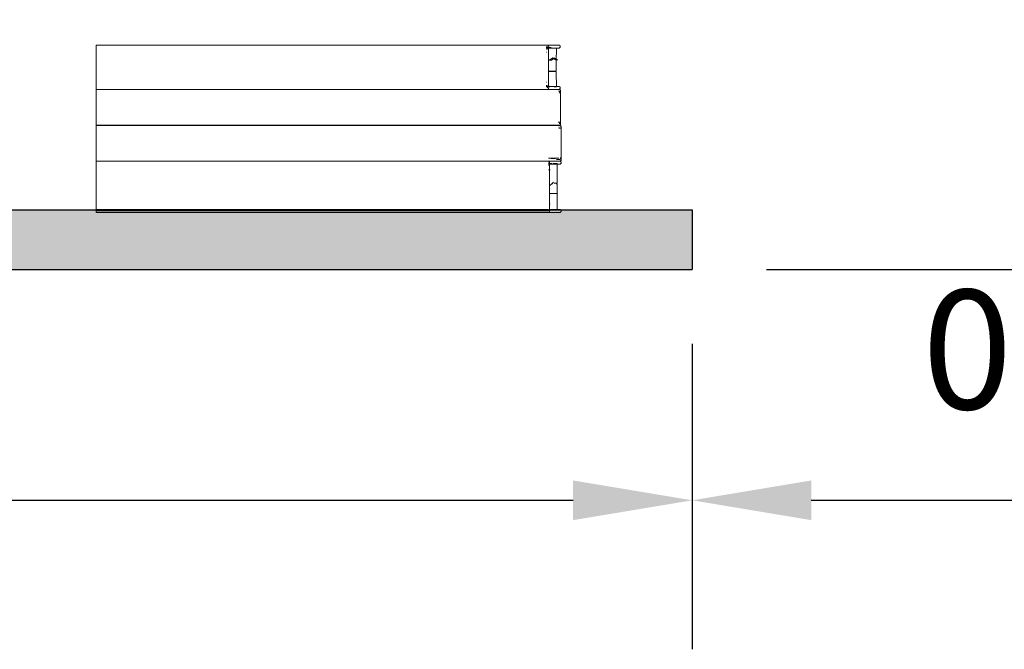
# Model space of a CAD drawing. Units: millimetres. Extents: x 7894 to 8038, y 6851 to 6951.
# Tile 25 of 49: x 7958.696 to 7966.961, y 6903.287 to 6908.569. Entities that reach past the tile are written whole.
import ezdxf

# ---------------------------------------------------------------- set-up
doc = ezdxf.new("R2010")
doc.units = ezdxf.units.MM
for name, color, linetype, lineweight in [('A-ANNO-DIMS', 2, 'Continuous', 18), ('A-FURN-BOOK', 8, 'Continuous', 13), ('A-FURN-SHLF', 7, 'Continuous', 30)]:
    doc.layers.add(name, color=color, linetype=linetype, lineweight=lineweight)
doc.layers.add('A-FURN-PATT', color=32, linetype='Continuous', lineweight=9, true_color=0xcd6928)
doc.styles.get("Standard").update_dxf_attribs({"font": 'arial.ttf'})
doc.dimstyles.new('ISO-25', dxfattribs={"dimtxt": 1, "dimasz": 1, "dimexe": 1.25, "dimexo": 0.625, "dimtad": 1, "dimdec": 0, "dimlunit": 4, "dimtxsty": 'Standard', "dimcen": 2.5, "dimclrt": 1, "dimadec": 0, "dimazin": 0, "dimtfac": 1, "dimtdec": 0, "dimtmove": 0, "dimatfit": 3, "dimfxl": 1, "dimarcsym": 0})

# ---------------------------------------------------------------- blocks, each defined once
blk = doc.blocks.new('*D23')
at = {"layer": 'A-ANNO-DIMS', "color": 0, "lineweight": -2, "transparency": 16777216}
for p, q in [((7940.0888, 6907.098), (7940.0888, 6947.7928)), ((7971.9356, 6928.989), (7971.9356, 6947.7928)), ((7941.0888, 6946.5428), (7970.9356, 6946.5428))]:
    blk.add_line(p, q, dxfattribs=at)
at = {"layer": 'A-ANNO-DIMS', "color": 0, "transparency": 16777216}
for points in [[(7941.0888, 6946.7095), (7941.0888, 6946.3762), (7940.0888, 6946.5428)], [(7970.9356, 6946.7095), (7970.9356, 6946.3762), (7971.9356, 6946.5428)]]:
    blk.add_solid(points, dxfattribs=at)
at = {"layer": 'Defpoints', "color": 0, "transparency": 16777216}
for p in [(7971.9356, 6946.5428), (7971.9356, 6928.364), (7940.0888, 6906.473)]:
    blk.add_point(p, dxfattribs=at)
at = {"layer": 'A-ANNO-DIMS', "color": 1, "transparency": 16777216, "insert": (7956.0122, 6947.6784), "char_height": 1, "attachment_point": 5}
blk.add_mtext('2\'-8"', dxfattribs=at)
blk = doc.blocks.new('*D25')
at = {"layer": 'A-ANNO-DIMS', "color": 0, "lineweight": -2, "transparency": 16777216}
for p, q in [((7940.0888, 6905.848), (7940.0888, 6903.2865)), ((7964.3408, 6905.8484), (7964.3408, 6903.2865)), ((7941.0888, 6904.5365), (7963.3408, 6904.5365))]:
    blk.add_line(p, q, dxfattribs=at)
at = {"layer": 'A-ANNO-DIMS', "color": 0, "transparency": 16777216}
for points in [[(7941.0888, 6904.7032), (7941.0888, 6904.3699), (7940.0888, 6904.5365)], [(7963.3408, 6904.7032), (7963.3408, 6904.3699), (7964.3408, 6904.5365)]]:
    blk.add_solid(points, dxfattribs=at)
at = {"layer": 'Defpoints', "color": 0, "transparency": 16777216}
for p in [(7940.0888, 6906.473), (7964.3408, 6906.4734), (7964.3408, 6904.5365)]:
    blk.add_point(p, dxfattribs=at)
at = {"layer": 'A-ANNO-DIMS', "color": 1, "transparency": 16777216, "insert": (7952.2148, 6905.6786), "char_height": 1, "attachment_point": 5}
blk.add_mtext('2\'-0 1/2"', dxfattribs=at)
blk = doc.blocks.new('*D26')
at = {"layer": 'A-ANNO-DIMS', "color": 0, "lineweight": -2, "transparency": 16777216}
for p, q in [((7950.9654, 6918.7198), (7975.2272, 6918.7198)), ((7973.9772, 6917.7198), (7973.9772, 6907.4734)), ((7964.9658, 6906.4734), (7975.2272, 6906.4734))]:
    blk.add_line(p, q, dxfattribs=at)
at = {"layer": 'A-ANNO-DIMS', "color": 0, "transparency": 16777216}
for points in [[(7973.8105, 6917.7198), (7974.1439, 6917.7198), (7973.9772, 6918.7198)], [(7973.8105, 6907.4734), (7974.1439, 6907.4734), (7973.9772, 6906.4734)]]:
    blk.add_solid(points, dxfattribs=at)
at = {"layer": 'Defpoints', "color": 0, "transparency": 16777216}
for p in [(7950.3404, 6918.7198), (7964.3408, 6906.4734), (7973.9772, 6906.4734)]:
    blk.add_point(p, dxfattribs=at)
at = {"layer": 'A-ANNO-DIMS', "color": 1, "transparency": 16777216, "insert": (7972.8416, 6912.5966), "char_height": 1, "attachment_point": 5, "rotation": 90}
blk.add_mtext('1\'-0"', dxfattribs=at)
blk = doc.blocks.new('*D34')
at = {"layer": 'A-ANNO-DIMS', "color": 0, "lineweight": -2, "transparency": 16777216}
for p, q in [((7971.2171, 6922.0033), (7971.2171, 6903.2865)), ((7964.3408, 6905.8484), (7964.3408, 6903.2865)), ((7965.3408, 6904.5365), (7970.2171, 6904.5365))]:
    blk.add_line(p, q, dxfattribs=at)
at = {"layer": 'A-ANNO-DIMS', "color": 0, "transparency": 16777216}
for points in [[(7965.3408, 6904.7032), (7965.3408, 6904.3699), (7964.3408, 6904.5365)], [(7970.2171, 6904.7032), (7970.2171, 6904.3699), (7971.2171, 6904.5365)]]:
    blk.add_solid(points, dxfattribs=at)
at = {"layer": 'Defpoints', "color": 0, "transparency": 16777216}
for p in [(7971.2171, 6922.6283), (7964.3408, 6906.4734), (7971.2171, 6904.5365)]:
    blk.add_point(p, dxfattribs=at)
at = {"layer": 'A-ANNO-DIMS', "color": 1, "transparency": 16777216, "insert": (7967.779, 6905.6721), "char_height": 1, "attachment_point": 5}
blk.add_mtext('0\'-7"', dxfattribs=at)

msp = doc.modelspace()

# ---------------------------------------------------------------- hatches: boundary and pattern name
at = {"layer": 'A-FURN-PATT'}
h = msp.add_hatch(color=256, dxfattribs=at)
h.dxf.hatch_style = 1
h.paths.add_polyline_path([(7942.8406, 6913.3629), (7942.8593, 6913.356), (7942.8677, 6913.356), (7942.8677, 6914.2132), (7942.876, 6914.2376), (7942.8813, 6914.2376), (7942.9022, 6914.2457), (7943.3657, 6914.2457), (7943.3844, 6914.2376), (7943.3861, 6914.2376), (7943.3858, 6914.2132), (7943.3852, 6913.2312), (7943.3944, 6906.9948), (7943.387, 6906.9732), (7943.4027, 6906.9732), (7943.403, 6906.9948), (7943.4029, 6908.4372), (7943.3944, 6914.2132), (7943.4169, 6914.2376), (7943.4198, 6914.2457), (7943.4555, 6914.2457), (7943.4603, 6914.238), (7943.8607, 6914.2452), (7943.8615, 6914.2457), (7943.8623, 6914.2452), (7943.8866, 6914.2457), (7943.8944, 6914.2402), (7943.9104, 6914.2376), (7943.9211, 6914.2132), (7943.9294, 6914.2376), (7943.9318, 6914.2376), (7943.9453, 6914.2398), (7943.9488, 6914.2457), (7943.9797, 6914.2452), (7943.9807, 6914.2457), (7943.9815, 6914.2451), (7944.3738, 6914.2376), (7944.3882, 6914.2457), (7944.4201, 6914.2457), (7944.4341, 6914.2376), (7944.4395, 6914.2376), (7944.4478, 6914.2132), (7944.4478, 6914.1031), (7944.4622, 6914.099), (7944.7359, 6914.1607), (7944.8923, 6914.2014), (7944.9541, 6914.2098), (7944.955, 6914.21), (7946.556, 6907.1325), (7946.5534, 6907.1122), (7946.5529, 6907.1152), (7946.499, 6907.103), (7946.3343, 6907.0604), (7946.0282, 6906.9914), (7945.6731, 6908.5712), (7944.4484, 6914.0015), (7944.4478, 6906.9948), (7944.4404, 6906.9732), (7947.0373, 6906.9734), (7964.3408, 6906.9734), (7964.3408, 6906.4734), (7947.0373, 6906.4734), (7940.0888, 6906.473), (7940.0888, 6906.973), (7941.9951, 6906.9731), (7941.9899, 6906.9898), (7941.9899, 6913.3353), (7941.9968, 6913.3574), (7942.003, 6913.3571), (7942.0169, 6913.3629), (7942.0366, 6913.3629), (7942.0378, 6913.3629), (7942.0479, 6913.356), (7942.8142, 6913.356), (7942.8157, 6913.356), (7942.8346, 6913.356)])
h.paths.add_polyline_path([(7942.8598, 6913.0201), (7942.861, 6913.3353), (7942.8677, 6906.9948), (7942.876, 6906.9759), (7942.876, 6906.9903), (7942.8813, 6914.2376), (7942.876, 6914.2321), (7942.876, 6914.2177), (7942.8809, 6906.9647), (7942.8784, 6906.9704), (7942.876, 6906.9704), (7942.8574, 6906.9704), (7942.8613, 6911.8549)], flags=16)
h.paths.add_polyline_path([(7942.8613, 6911.8549), (7942.8677, 6906.9948), (7942.8686, 6906.9921), (7942.8677, 6906.9898), (7942.8616, 6906.9704), (7942.8598, 6906.9704), (7942.8574, 6906.9704), (7942.0002, 6906.9704), (7941.9978, 6906.9704), (7941.996, 6906.9704), (7941.9899, 6906.9898), (7941.9978, 6906.9704), (7942.0002, 6906.9704), (7942.8598, 6906.9704), (7942.8616, 6906.9748)], flags=16)
h.paths.add_polyline_path([(7942.023, 6913.356), (7942.0169, 6913.3629), (7942.0366, 6913.3629), (7942.0378, 6913.3629), (7942.0367, 6913.3614), (7942.0369, 6913.356)], flags=16)
h.paths.add_polyline_path([(7942.0366, 6913.3629), (7942.0169, 6913.3629), (7942.0196, 6913.3598)], flags=0)
h.paths.add_polyline_path([(7942.0353, 6913.356), (7942.0369, 6913.356), (7942.0367, 6913.3614)], flags=0)
h.paths.add_polyline_path([(7943.9293, 6906.9759), (7943.9211, 6906.9948), (7943.9294, 6906.9704)], flags=0)
h.paths.add_polyline_path([(7943.9125, 6914.2132), (7943.8982, 6914.2376), (7943.8944, 6914.2402), (7943.8832, 6914.2421), (7943.8781, 6914.2367), (7943.8765, 6914.2376), (7943.8789, 6914.2376), (7943.8866, 6914.2457), (7943.8623, 6914.2452), (7943.8607, 6914.2452), (7943.8615, 6914.2457), (7943.8623, 6914.2452), (7943.8866, 6914.2457), (7943.8944, 6914.2402), (7943.8982, 6914.2376), (7943.9097, 6914.218), (7943.9125, 6914.2168), (7943.9079, 6906.9704), (7943.9104, 6906.9704), (7943.9211, 6914.2132), (7943.9294, 6914.2376), (7943.9318, 6914.2376), (7943.9453, 6914.2398), (7943.9488, 6914.2457), (7943.9797, 6914.2452), (7943.9807, 6914.2457), (7943.9815, 6914.2451), (7944.3738, 6914.2376), (7944.3882, 6914.2457), (7944.4201, 6914.2457), (7944.4341, 6914.2376), (7944.4395, 6914.2376), (7944.4395, 6914.2177), (7944.4341, 6914.0941), (7944.4478, 6914.1004), (7944.4513, 6914.1021), (7944.4622, 6914.099), (7944.4343, 6914.0927), (7944.429, 6914.0915), (7944.4341, 6914.069), (7944.4484, 6914.0015), (7944.4341, 6914.0649), (7944.4346, 6906.9704), (7944.4371, 6906.9704), (7944.4395, 6906.9759), (7944.4395, 6906.9704), (7943.931, 6906.9704), (7943.9128, 6906.9704), (7943.9079, 6906.9704)], flags=16)
h.paths.add_polyline_path([(7943.9211, 6914.2132), (7943.9294, 6914.2376), (7943.9318, 6914.2376), (7943.9453, 6914.2398), (7943.9488, 6914.2457), (7943.9797, 6914.2452), (7943.9807, 6914.2457), (7943.9815, 6914.2451), (7944.3738, 6914.2376), (7944.3882, 6914.2457), (7944.4201, 6914.2457), (7944.4321, 6914.2387), (7944.4249, 6914.2376), (7944.4041, 6914.2376), (7944.4032, 6914.2136), (7944.4032, 6914.2376), (7944.4025, 6914.2379), (7944.3897, 6914.2382), (7944.3753, 6914.2384), (7944.3738, 6914.2376), (7943.9815, 6914.2451), (7943.9488, 6914.2457), (7943.9453, 6914.2398), (7943.9294, 6914.2132), (7943.931, 6906.9721), (7943.931, 6906.9704), (7943.9294, 6906.9704), (7943.9293, 6906.9759), (7943.9294, 6914.2132), (7943.9439, 6914.2376), (7943.9318, 6914.2376)], flags=0)
h.paths.add_polyline_path([(7942.8813, 6914.2376), (7942.8778, 6914.2362), (7942.8796, 6914.2404), (7942.885, 6914.239)], flags=17)
h.paths.add_polyline_path([(7944.4116, 6914.242), (7944.4104, 6914.2408), (7944.4125, 6914.2418)], flags=0)
h.paths.add_polyline_path([(7944.3879, 6914.2382), (7944.3882, 6914.2457), (7944.4094, 6914.241), (7944.4103, 6914.2408), (7944.4036, 6914.2373), (7944.39, 6914.2447), (7944.3897, 6914.2382)], flags=0)
h.paths.add_polyline_path([(7963.1359, 6906.9526), (7963.1396, 6906.9526), (7963.1431, 6906.9582)], flags=16)
h.paths.add_polyline_path([(7954.3975, 6907.3902), (7954.397, 6907.3948), (7954.3984, 6907.4007), (7954.3975, 6907.567), (7954.3984, 6907.5978), (7954.3986, 6907.7694), (7954.3978, 6907.7989), (7954.399, 6907.8759), (7954.3992, 6907.9037), (7954.3944, 6907.9081), (7954.4019, 6907.9055), (7954.3996, 6907.93), (7954.3988, 6907.9307), (7954.3841, 6907.9429), (7946.6754, 6907.9429), (7946.6535, 6907.9232), (7946.6531, 6907.9127), (7946.6527, 6907.7694), (7946.6525, 6907.4007), (7946.653, 6907.1185), (7946.6574, 6907.1224), (7946.656, 6907.1145), (7946.6571, 6907.1135), (7946.6675, 6907.1209), (7946.7515, 6907.1209), (7946.9105, 6907.1209), (7954.3003, 6907.1209), (7954.3895, 6907.1209), (7954.3915, 6907.1191), (7954.3991, 6907.1209), (7954.399, 6907.1383), (7954.3978, 6907.2163), (7954.3986, 6907.2413)], flags=17)
h.paths.add_polyline_path([(7954.3003, 6907.1209), (7954.3003, 6907.1136), (7946.9105, 6907.1129), (7946.7516, 6907.1136), (7946.7515, 6907.1209), (7946.6675, 6907.1209), (7946.6531, 6907.1106), (7946.653, 6907.1185), (7946.6574, 6907.1224), (7946.656, 6907.1145), (7946.6571, 6907.1135), (7946.6675, 6907.1209), (7946.7515, 6907.1209), (7946.9105, 6907.1209)], flags=17)
h.paths.add_polyline_path([(7954.3981, 6907.9048), (7954.3944, 6907.9081), (7954.3997, 6907.9062), (7954.4007, 6907.9186), (7954.4019, 6907.9055), (7954.405, 6907.9072), (7954.4044, 6907.9046), (7954.4027, 6907.8974), (7954.4024, 6907.9009), (7954.3996, 6907.9034), (7954.3996, 6907.9025), (7954.3994, 6907.9023), (7954.3995, 6907.9035)], flags=17)

# ---------------------------------------------------------------- linework, layer by layer
at = {"layer": 'A-FURN-BOOK'}
for p, q in [((7963.1286, 6908.3556), (7959.3384, 6908.3556)), ((7959.3384, 6906.9526), (7959.3384, 6908.3556)), ((7963.1316, 6908.353), (7963.1286, 6908.3556)), ((7963.2254, 6908.3556), (7963.1286, 6908.3556)), ((7963.1316, 6908.353), (7963.1358, 6908.35)), ((7963.1358, 6908.3494), (7963.1358, 6908.35)), ((7963.1363, 6908.349), (7963.1358, 6908.3494)), ((7963.1367, 6908.3434), (7963.1363, 6908.349)), ((7963.2254, 6908.3556), (7963.233, 6908.3486)), ((7963.233, 6908.3486), (7963.233, 6908.3376)), ((7963.1299, 6908.3414), (7963.1163, 6908.3414)), ((7963.1172, 6908.3363), (7963.1163, 6908.3366)), ((7963.1163, 6908.3305), (7963.1276, 6908.3305)), ((7963.1183, 6908.3228), (7963.1163, 6908.3228)), ((7963.1169, 6908.2977), (7963.1163, 6908.2977)), ((7963.1324, 6908.3366), (7963.1172, 6908.3363)), ((7963.1287, 6908.3295), (7963.1276, 6908.3295)), ((7963.1299, 6908.3228), (7963.1276, 6908.3228)), ((7963.1293, 6908.3299), (7963.1287, 6908.3295)), ((7963.1336, 6908.338), (7963.1299, 6908.3414)), ((7963.1359, 6908.3283), (7963.1299, 6908.3228)), ((7963.1354, 6908.3363), (7963.1362, 6908.3364)), ((7963.1362, 6908.3356), (7963.1354, 6908.3363)), ((7963.1362, 6908.3352), (7963.1354, 6908.3346)), ((7963.1354, 6908.3305), (7963.1362, 6908.3352)), ((7963.1359, 6908.3298), (7963.1354, 6908.3305)), ((7963.136, 6908.3305), (7963.1354, 6908.3305)), ((7963.1354, 6908.2332), (7963.1358, 6908.2861)), ((7963.1358, 6908.2861), (7963.1359, 6908.3217)), ((7963.1359, 6908.3283), (7963.1359, 6908.3298)), ((7963.1375, 6908.3298), (7963.1359, 6908.3283)), ((7963.1359, 6908.3217), (7963.1359, 6908.3283)), ((7963.1378, 6908.3301), (7963.136, 6908.3305)), ((7963.1362, 6908.3364), (7963.1367, 6908.3434)), ((7963.1362, 6908.3364), (7963.1373, 6908.3367)), ((7963.1362, 6908.3356), (7963.1362, 6908.3364)), ((7963.1375, 6908.3344), (7963.1362, 6908.3356)), ((7963.1362, 6908.3352), (7963.1362, 6908.3356)), ((7963.1373, 6908.3367), (7963.1367, 6908.3434)), ((7963.1388, 6908.3376), (7963.1373, 6908.3367)), ((7963.1373, 6908.3367), (7963.1386, 6908.3365)), ((7963.1375, 6908.3344), (7963.1373, 6908.3367)), ((7963.1375, 6908.3298), (7963.1378, 6908.3301)), ((7963.1378, 6908.3301), (7963.138, 6908.3319)), ((7963.1378, 6908.3301), (7963.1405, 6908.3305)), ((7963.138, 6908.3319), (7963.1384, 6908.3357)), ((7963.1384, 6908.3357), (7963.1386, 6908.3365)), ((7963.1386, 6908.3365), (7963.1388, 6908.3376)), ((7963.1386, 6908.3365), (7963.1402, 6908.3366)), ((7963.1405, 6908.3305), (7963.2012, 6908.3305)), ((7963.1443, 6908.3364), (7963.1427, 6908.3366)), ((7963.1583, 6908.3366), (7963.1443, 6908.3364)), ((7963.2009, 6908.2977), (7963.2006, 6908.2549)), ((7963.2012, 6908.3305), (7963.2009, 6908.2977)), ((7963.2012, 6908.3305), (7963.2254, 6908.3305)), ((7963.233, 6908.3376), (7963.2254, 6908.3305)), ((7963.1358, 6908.2327), (7963.1354, 6908.2332)), ((7963.1354, 6908.2327), (7963.1354, 6908.2332)), ((7963.1354, 6908.2327), (7963.1358, 6908.2327)), ((7963.1354, 6908.2314), (7963.1354, 6908.2327)), ((7963.1354, 6908.2314), (7963.1358, 6908.2314)), ((7963.1354, 6908.2307), (7963.1354, 6908.2314)), ((7963.1354, 6908.2307), (7963.1467, 6908.2308)), ((7963.1354, 6908.2295), (7963.1354, 6908.2307)), ((7963.1354, 6908.2295), (7963.1358, 6908.229)), ((7963.1354, 6908.229), (7963.1354, 6908.2295)), ((7963.1358, 6908.229), (7963.1354, 6908.229)), ((7963.1358, 6908.2103), (7963.1354, 6908.229)), ((7963.1354, 6908.1368), (7963.1358, 6908.2103)), ((7963.1431, 6908.2332), (7963.1358, 6908.2327)), ((7963.1358, 6908.2314), (7963.1467, 6908.2308)), ((7963.1436, 6908.2291), (7963.1358, 6908.229)), ((7963.1431, 6908.2332), (7963.1436, 6908.2328)), ((7963.1436, 6908.2328), (7963.1444, 6908.2332)), ((7963.1444, 6908.2295), (7963.1436, 6908.2291)), ((7963.145, 6908.2332), (7963.1444, 6908.2332)), ((7963.1588, 6908.2309), (7963.1444, 6908.2295)), ((7963.1467, 6908.2308), (7963.1444, 6908.2295)), ((7963.145, 6908.2332), (7963.1707, 6908.2484)), ((7963.1467, 6908.2308), (7963.1472, 6908.2314)), ((7963.1588, 6908.2309), (7963.1472, 6908.2314)), ((7963.1707, 6908.2446), (7963.1585, 6908.2376)), ((7963.1588, 6908.2309), (7963.177, 6908.2414)), ((7963.1859, 6908.2465), (7963.1707, 6908.2484)), ((7963.1707, 6908.2484), (7963.1766, 6908.2453)), ((7963.1766, 6908.2453), (7963.1707, 6908.2446)), ((7963.1743, 6908.2427), (7963.1707, 6908.2446)), ((7963.1859, 6908.2465), (7963.1766, 6908.2453)), ((7963.1766, 6908.2453), (7963.1789, 6908.2442)), ((7963.177, 6908.2414), (7963.1805, 6908.2434)), ((7963.1931, 6908.2332), (7963.177, 6908.2414)), ((7963.1805, 6908.2434), (7963.1859, 6908.2465)), ((7963.1805, 6908.2434), (7963.1948, 6908.2362)), ((7963.2006, 6908.2382), (7963.1859, 6908.2465)), ((7963.1973, 6908.2332), (7963.1931, 6908.2332)), ((7963.1968, 6908.2314), (7963.1931, 6908.2332)), ((7963.1968, 6908.2314), (7963.1989, 6908.2314)), ((7963.2005, 6908.2295), (7963.1968, 6908.2314)), ((7963.2126, 6908.2314), (7963.2005, 6908.2295)), ((7963.2005, 6908.2295), (7963.2005, 6908.2078)), ((7963.2005, 6908.1368), (7963.2005, 6908.2078)), ((7963.2006, 6908.2549), (7963.2006, 6908.2382)), ((7963.2126, 6908.2314), (7963.2006, 6908.2382)), ((7963.1354, 6908.133), (7963.1354, 6908.1368)), ((7963.1354, 6908.1368), (7963.1436, 6908.1368)), ((7963.1358, 6908.1255), (7963.1354, 6908.133)), ((7963.1358, 6908.133), (7963.1354, 6908.133)), ((7963.1358, 6908.133), (7963.1436, 6908.1331)), ((7963.1358, 6908.1255), (7963.1359, 6908.0187)), ((7963.1436, 6908.1368), (7963.2005, 6908.1368)), ((7963.1436, 6908.1331), (7963.2005, 6908.133)), ((7963.2005, 6908.1368), (7963.1763, 6908.1349)), ((7963.1763, 6908.1349), (7963.2005, 6908.133)), ((7963.2006, 6908.0878), (7963.2005, 6908.133)), ((7963.1163, 6908.0451), (7963.1169, 6908.0451)), ((7963.1256, 6908.0177), (7963.1163, 6908.0177)), ((7963.1359, 6908.0121), (7963.1359, 6908.0187)), ((7963.2006, 6908.0878), (7963.2009, 6908.0451)), ((7963.2009, 6908.0451), (7963.2018, 6908.0099)), ((7963.1286, 6907.9848), (7959.3384, 6907.9848)), ((7963.2269, 6907.9836), (7959.4277, 6907.9836)), ((7963.1278, 6908.0109), (7963.1163, 6908.0109)), ((7963.1163, 6908.0099), (7963.1301, 6908.0099)), ((7963.1191, 6908.0064), (7963.1323, 6908.0061)), ((7963.1323, 6908.0061), (7963.1193, 6908.0061)), ((7963.1291, 6907.999), (7963.1251, 6907.999)), ((7963.1286, 6907.9848), (7963.1358, 6907.9905)), ((7963.1286, 6907.9848), (7963.2254, 6907.9848)), ((7963.1301, 6908.0099), (7963.1293, 6908.0105)), ((7963.1312, 6908.0099), (7963.1301, 6908.0099)), ((7963.1312, 6908.0099), (7963.1332, 6908.008)), ((7963.133, 6908.0076), (7963.1312, 6908.0099)), ((7963.1341, 6908.0099), (7963.1312, 6908.0099)), ((7963.1359, 6908.0121), (7963.1352, 6908.0128)), ((7963.1354, 6908.0099), (7963.1359, 6908.0106)), ((7963.136, 6908.0099), (7963.1354, 6908.0099)), ((7963.1354, 6908.0063), (7963.1354, 6908.0099)), ((7963.1354, 6908.0063), (7963.1362, 6908.006)), ((7963.1362, 6908.006), (7963.1354, 6908.006)), ((7963.1362, 6908.0048), (7963.1354, 6908.0041)), ((7963.1358, 6907.9905), (7963.1363, 6907.9913)), ((7963.1359, 6908.0106), (7963.1359, 6908.0121)), ((7963.1375, 6908.0106), (7963.1359, 6908.0121)), ((7963.1378, 6908.0103), (7963.136, 6908.0099)), ((7963.1362, 6908.0052), (7963.1362, 6908.006)), ((7963.1375, 6908.006), (7963.1362, 6908.0052)), ((7963.1375, 6908.006), (7963.1362, 6908.006)), ((7963.1362, 6908.0052), (7963.1362, 6908.0048)), ((7963.1362, 6908.0048), (7963.1367, 6907.9965)), ((7963.1362, 6908.0048), (7963.1373, 6908.0039)), ((7963.1363, 6907.9913), (7963.1367, 6907.9965)), ((7963.1367, 6907.9965), (7963.1373, 6908.0039)), ((7963.1373, 6908.0039), (7963.1375, 6908.006)), ((7963.1373, 6908.0039), (7963.1388, 6908.0028)), ((7963.1378, 6908.0103), (7963.1375, 6908.0106)), ((7963.1405, 6908.0099), (7963.1378, 6908.0103)), ((7963.138, 6908.0084), (7963.1378, 6908.0103)), ((7963.1384, 6908.0048), (7963.138, 6908.0084)), ((7963.1388, 6908.0028), (7963.1384, 6908.0048)), ((7963.2018, 6908.0099), (7963.1405, 6908.0099)), ((7963.182, 6908.0062), (7963.1825, 6908.0061)), ((7963.2013, 6908.0061), (7963.1825, 6908.0061)), ((7963.2018, 6908.0099), (7963.2013, 6908.0061)), ((7963.2018, 6908.0099), (7963.2254, 6908.0099)), ((7963.2269, 6907.9698), (7963.2182, 6907.9698)), ((7963.2254, 6908.0099), (7963.233, 6908.0028)), ((7963.233, 6907.9918), (7963.2254, 6907.9848)), ((7963.2269, 6907.9836), (7963.2345, 6907.9768)), ((7963.2345, 6907.9772), (7963.2269, 6907.9836)), ((7963.2269, 6907.9836), (7963.2345, 6907.9781)), ((7963.2326, 6907.9646), (7963.2269, 6907.9698)), ((7963.2326, 6907.9646), (7963.2269, 6907.9592)), ((7963.2341, 6907.9633), (7963.2269, 6907.9582)), ((7963.2345, 6907.9584), (7963.2269, 6907.9516)), ((7963.2345, 6907.9663), (7963.2326, 6907.9646)), ((7963.2341, 6907.9633), (7963.2326, 6907.9646)), ((7963.233, 6908.0028), (7963.233, 6907.9918)), ((7963.2341, 6907.9633), (7963.2345, 6907.9642)), ((7963.2345, 6907.9636), (7963.2341, 6907.9633)), ((7963.2345, 6907.9629), (7963.2341, 6907.9633)), ((7963.2345, 6907.9772), (7963.2345, 6907.9781)), ((7963.2345, 6907.9768), (7963.2345, 6907.9772)), ((7963.2345, 6907.9663), (7963.2345, 6907.9768)), ((7963.2345, 6907.9642), (7963.2345, 6907.9663)), ((7963.2345, 6907.9642), (7963.2345, 6907.9636)), ((7963.2345, 6907.9636), (7963.2345, 6907.9629)), ((7963.2345, 6907.9632), (7963.2345, 6907.9636)), ((7963.2345, 6907.9629), (7963.2345, 6907.9632)), ((7963.2345, 6907.9584), (7963.2345, 6907.9629)), ((7963.2345, 6907.9584), (7963.2345, 6907.6896)), ((7963.2156, 6907.7085), (7963.2269, 6907.7085)), ((7963.2269, 6907.6979), (7963.2243, 6907.6979)), ((7963.2282, 6907.7149), (7963.2269, 6907.716)), ((7963.2269, 6907.7085), (7963.2313, 6907.7045)), ((7963.2293, 6907.7001), (7963.2269, 6907.6979)), ((7963.2345, 6907.6896), (7963.2269, 6907.684)), ((7963.232, 6907.7058), (7963.2278, 6907.7088)), ((7963.2338, 6907.7098), (7963.2328, 6907.7107)), ((7963.2269, 6907.684), (7959.3384, 6907.684)), ((7959.3384, 6907.6826), (7963.2304, 6907.6826)), ((7963.2253, 6907.6687), (7963.2228, 6907.6687)), ((7963.2304, 6907.6582), (7963.2229, 6907.6582)), ((7963.2304, 6907.6826), (7963.2337, 6907.6796)), ((7963.2336, 6907.6826), (7963.2304, 6907.6826)), ((7963.2336, 6907.6826), (7963.2411, 6907.677)), ((7963.2349, 6907.6579), (7963.2343, 6907.6581)), ((7963.2349, 6907.6579), (7963.2393, 6907.6619)), ((7963.2391, 6907.6624), (7963.2379, 6907.6631)), ((7963.2382, 6907.6749), (7963.2385, 6907.6727)), ((7963.2393, 6907.6574), (7963.2383, 6907.6565)), ((7963.2385, 6907.6727), (7963.2387, 6907.6692)), ((7963.239, 6907.6645), (7963.2391, 6907.6624)), ((7963.2391, 6907.6624), (7963.2393, 6907.6619)), ((7963.2393, 6907.6619), (7963.2402, 6907.6618)), ((7963.2396, 6907.6587), (7963.2393, 6907.6574)), ((7963.2402, 6907.6618), (7963.2396, 6907.6587)), ((7963.2404, 6907.6626), (7963.2402, 6907.6618)), ((7963.2404, 6907.6626), (7963.2408, 6907.6668)), ((7963.2408, 6907.668), (7963.2411, 6907.677)), ((7963.2411, 6907.677), (7963.2414, 6907.6677)), ((7963.2414, 6907.6677), (7963.2416, 6907.6208)), ((7963.2416, 6907.6208), (7963.2417, 6907.5641)), ((7963.2417, 6907.5641), (7963.2417, 6907.4991)), ((7963.2417, 6907.4991), (7963.2415, 6907.4103)), ((7959.3384, 6907.3817), (7963.1359, 6907.3817)), ((7963.2336, 6907.383), (7959.6826, 6907.383)), ((7963.1932, 6907.4074), (7963.1338, 6907.4074)), ((7963.136, 6907.3562), (7963.1348, 6907.3562)), ((7963.1372, 6907.3678), (7963.1349, 6907.3678)), ((7963.1393, 6907.3627), (7963.1349, 6907.3626)), ((7963.1389, 6907.3791), (7963.1359, 6907.3817)), ((7963.1359, 6907.3817), (7963.2327, 6907.3817)), ((7963.1366, 6907.3566), (7963.136, 6907.3562)), ((7963.1409, 6907.3646), (7963.1372, 6907.3678)), ((7963.1427, 6907.3759), (7963.1389, 6907.3791)), ((7963.1389, 6907.3791), (7963.1431, 6907.3761)), ((7963.1435, 6907.3622), (7963.1427, 6907.3629)), ((7963.1435, 6907.3629), (7963.1427, 6907.3629)), ((7963.1435, 6907.3618), (7963.1427, 6907.3612)), ((7963.1427, 6907.3573), (7963.1435, 6907.3618)), ((7963.1432, 6907.3565), (7963.1427, 6907.3573)), ((7963.1433, 6907.3573), (7963.1427, 6907.3573)), ((7963.1435, 6907.3752), (7963.1431, 6907.3761)), ((7963.1431, 6907.3757), (7963.1431, 6907.3761)), ((7963.1435, 6907.3752), (7963.1431, 6907.3757)), ((7963.1432, 6907.3551), (7963.1432, 6907.3565)), ((7963.1448, 6907.3565), (7963.1432, 6907.3551)), ((7963.145, 6907.3568), (7963.1433, 6907.3573)), ((7963.144, 6907.3697), (7963.1435, 6907.3752)), ((7963.1435, 6907.3629), (7963.144, 6907.3697)), ((7963.1446, 6907.3633), (7963.1435, 6907.3629)), ((7963.1435, 6907.3629), (7963.1435, 6907.3622)), ((7963.1448, 6907.361), (7963.1435, 6907.3622)), ((7963.1435, 6907.3618), (7963.1435, 6907.3622)), ((7963.1446, 6907.3633), (7963.144, 6907.3697)), ((7963.1461, 6907.3641), (7963.1446, 6907.3633)), ((7963.1458, 6907.3629), (7963.1446, 6907.3633)), ((7963.1448, 6907.361), (7963.1446, 6907.3633)), ((7963.1448, 6907.3565), (7963.145, 6907.3568)), ((7963.145, 6907.3568), (7963.1452, 6907.3586)), ((7963.159, 6907.3573), (7963.145, 6907.3568)), ((7963.1452, 6907.3586), (7963.1457, 6907.3622)), ((7963.1457, 6907.3622), (7963.1458, 6907.3629)), ((7963.1458, 6907.3629), (7963.1461, 6907.3641)), ((7963.1509, 6907.3627), (7963.1458, 6907.3629)), ((7963.1653, 6907.3629), (7963.1509, 6907.3627)), ((7963.1931, 6907.4039), (7963.1581, 6907.4037)), ((7963.2078, 6907.3573), (7963.159, 6907.3573)), ((7963.1742, 6907.3629), (7963.1748, 6907.3628)), ((7963.2078, 6907.3629), (7963.1748, 6907.3628)), ((7963.1932, 6907.4074), (7963.1931, 6907.4039)), ((7963.2229, 6907.4074), (7963.1932, 6907.4074)), ((7963.2315, 6907.3969), (7963.2026, 6907.3969)), ((7963.2078, 6907.3573), (7963.2075, 6907.3108)), ((7963.2078, 6907.3629), (7963.2078, 6907.3573)), ((7963.2078, 6907.3573), (7963.2327, 6907.3573)), ((7963.2337, 6907.386), (7963.2321, 6907.3845)), ((7963.2327, 6907.3817), (7963.2403, 6907.3748)), ((7963.2403, 6907.3641), (7963.2327, 6907.3573)), ((7963.2411, 6907.3885), (7963.2336, 6907.383)), ((7963.2393, 6907.4037), (7963.2341, 6907.4076)), ((7963.2391, 6907.4032), (7963.2341, 6907.399)), ((7963.2393, 6907.4082), (7963.235, 6907.412)), ((7963.238, 6907.3898), (7963.2365, 6907.3884)), ((7963.2383, 6907.392), (7963.238, 6907.3898)), ((7963.2389, 6907.3999), (7963.2387, 6907.3963)), ((7963.2391, 6907.4032), (7963.2389, 6907.3999)), ((7963.2393, 6907.4037), (7963.2391, 6907.4032)), ((7963.2393, 6907.4082), (7963.2395, 6907.4069)), ((7963.2404, 6907.4035), (7963.2393, 6907.4037)), ((7963.2395, 6907.4069), (7963.2401, 6907.4043)), ((7963.2401, 6907.4043), (7963.2404, 6907.4035)), ((7963.2403, 6907.3748), (7963.2403, 6907.3641)), ((7963.2404, 6907.4035), (7963.2407, 6907.4029)), ((7963.2407, 6907.4029), (7963.2408, 6907.3975)), ((7963.2414, 6907.3979), (7963.2408, 6907.3975)), ((7963.2411, 6907.3885), (7963.2408, 6907.3975)), ((7963.2415, 6907.4103), (7963.2414, 6907.3979)), ((7963.1367, 6907.3108), (7963.1347, 6907.3108)), ((7963.1372, 6907.3497), (7963.1348, 6907.3497)), ((7963.1432, 6907.3551), (7963.1372, 6907.3497)), ((7963.1426, 6907.3108), (7963.1432, 6907.3487)), ((7963.143, 6907.2963), (7963.1426, 6907.3108)), ((7963.1498, 6907.3108), (7963.1426, 6907.3108)), ((7963.1429, 6907.2118), (7963.143, 6907.2963)), ((7963.1432, 6907.3487), (7963.1432, 6907.3551)), ((7963.2075, 6907.3108), (7963.2072, 6907.2557)), ((7963.1424, 6907.1974), (7963.1429, 6907.2118)), ((7963.1424, 6907.1926), (7963.1424, 6907.1974)), ((7963.1424, 6907.1974), (7963.1442, 6907.1974)), ((7963.1429, 6907.1148), (7963.1424, 6907.1926)), ((7963.1461, 6907.1926), (7963.1424, 6907.1926)), ((7963.1627, 6907.1926), (7963.1502, 6907.1794)), ((7963.1627, 6907.1926), (7963.161, 6907.1926)), ((7963.1684, 6907.1974), (7963.1627, 6907.1926)), ((7963.1627, 6907.1926), (7963.1674, 6907.1974)), ((7963.1685, 6907.1926), (7963.1646, 6907.1926)), ((7963.1659, 6907.1974), (7963.1674, 6907.1974)), ((7963.1674, 6907.1974), (7963.1732, 6907.2034)), ((7963.1772, 6907.2058), (7963.1684, 6907.1974)), ((7963.1684, 6907.1974), (7963.1735, 6907.1974)), ((7963.171, 6907.1926), (7963.1703, 6907.1926)), ((7963.1772, 6907.2058), (7963.1732, 6907.2034)), ((7963.1816, 6907.1974), (7963.2071, 6907.1974)), ((7963.207, 6907.1926), (7963.1987, 6907.1926)), ((7963.2071, 6907.1974), (7963.2018, 6907.195)), ((7963.2018, 6907.195), (7963.207, 6907.1926)), ((7963.207, 6907.1399), (7963.207, 6907.1926)), ((7963.2071, 6907.1974), (7963.2072, 6907.2557)), ((7963.1422, 6907.1119), (7963.1429, 6907.1148)), ((7963.1425, 6907.1095), (7963.1422, 6907.1119)), ((7963.1502, 6907.1119), (7963.1422, 6907.1119)), ((7963.1425, 6907.1071), (7963.1425, 6907.1095)), ((7963.2105, 6907.1095), (7963.1425, 6907.1095)), ((7963.1475, 6907.177), (7963.1502, 6907.1794)), ((7963.2071, 6907.1119), (7963.181, 6907.1119)), ((7963.207, 6907.1399), (7963.2071, 6907.1119)), ((7963.2071, 6907.1119), (7963.2105, 6907.1095)), ((7963.2071, 6907.1071), (7963.2105, 6907.1095)), ((7963.143, 6907.0363), (7963.1425, 6907.1071)), ((7963.1425, 6907.1071), (7963.1496, 6907.1071)), ((7963.1426, 6907.024), (7963.143, 6907.0363)), ((7963.2072, 6907.0791), (7963.2071, 6907.1071)), ((7963.2072, 6907.0791), (7963.2075, 6907.024)), ((7963.0946, 6906.9771), (7959.3384, 6906.9771)), ((7963.0946, 6906.9735), (7959.3384, 6906.9731)), ((7963.1349, 6906.9665), (7959.3384, 6906.9665)), ((7963.1359, 6906.9526), (7959.3384, 6906.9526)), ((7963.0946, 6906.9771), (7963.0946, 6906.9735)), ((7963.1349, 6906.9771), (7963.0946, 6906.9771)), ((7963.0946, 6906.9735), (7963.1238, 6906.9734)), ((7963.1238, 6906.9734), (7963.1349, 6906.9731)), ((7963.1359, 6906.9526), (7963.1431, 6906.9582)), ((7963.1359, 6906.9526), (7963.2327, 6906.9526)), ((7963.1372, 6906.9665), (7963.1364, 6906.9665)), ((7963.1435, 6906.9726), (7963.1372, 6906.9665)), ((7963.1395, 6906.9731), (7963.1429, 6906.9731)), ((7963.1429, 6906.9731), (7963.1403, 6906.9749)), ((7963.1405, 6906.9753), (7963.1429, 6906.9731)), ((7963.1433, 6906.9771), (7963.1413, 6906.9771)), ((7963.1432, 6906.9856), (7963.1426, 6907.024)), ((7963.1426, 6907.024), (7963.1498, 6907.024)), ((7963.1432, 6906.9792), (7963.1426, 6906.9798)), ((7963.1429, 6906.9731), (7963.1433, 6906.9771)), ((7963.1435, 6906.9726), (7963.1429, 6906.9731)), ((7963.1431, 6906.9582), (7963.1436, 6906.9589)), ((7963.1432, 6906.9792), (7963.1432, 6906.9856)), ((7963.1432, 6906.9778), (7963.1432, 6906.9792)), ((7963.1448, 6906.9778), (7963.1432, 6906.9792)), ((7963.1433, 6906.9771), (7963.1432, 6906.9778)), ((7963.145, 6906.9775), (7963.1433, 6906.9771)), ((7963.1448, 6906.9733), (7963.1435, 6906.9726)), ((7963.1435, 6906.9726), (7963.1435, 6906.9721)), ((7963.1435, 6906.9726), (7963.1446, 6906.9712)), ((7963.1457, 6906.9721), (7963.1435, 6906.9726)), ((7963.1435, 6906.9721), (7963.144, 6906.9641)), ((7963.1436, 6906.9589), (7963.144, 6906.9641)), ((7963.144, 6906.9641), (7963.1446, 6906.9712)), ((7963.1446, 6906.9712), (7963.1448, 6906.9733)), ((7963.1446, 6906.9712), (7963.1461, 6906.9702)), ((7963.145, 6906.9775), (7963.1448, 6906.9778)), ((7963.1448, 6906.9733), (7963.1456, 6906.9731)), ((7963.159, 6906.9771), (7963.145, 6906.9775)), ((7963.1453, 6906.9756), (7963.145, 6906.9775)), ((7963.1456, 6906.9731), (7963.1453, 6906.9756)), ((7963.1456, 6906.9731), (7963.1509, 6906.9733)), ((7963.1457, 6906.9721), (7963.1456, 6906.9731)), ((7963.1779, 6906.9732), (7963.1457, 6906.9721)), ((7963.1461, 6906.9702), (7963.1457, 6906.9721)), ((7963.1509, 6906.9733), (7963.1779, 6906.9732)), ((7963.159, 6906.9771), (7963.2078, 6906.9771)), ((7963.1779, 6906.9732), (7963.2078, 6906.9731)), ((7963.2075, 6907.024), (7963.2078, 6906.9771)), ((7963.2078, 6906.9771), (7963.2078, 6906.9731)), ((7963.2078, 6906.9771), (7963.2327, 6906.9771)), ((7963.2327, 6906.9771), (7963.2403, 6906.9702)), ((7963.2403, 6906.9595), (7963.2327, 6906.9526)), ((7963.2403, 6906.9702), (7963.2403, 6906.9595))]:
    msp.add_line(p, q, dxfattribs=at)
at = {"layer": 'A-FURN-SHLF'}
for p, q in [((7947.0373, 6906.9734), (7964.3408, 6906.9734)), ((7964.3408, 6906.9734), (7964.3408, 6906.4734)), ((7947.0373, 6906.4734), (7964.3408, 6906.4734))]:
    msp.add_line(p, q, dxfattribs=at)

# ---------------------------------------------------------------- dimensions: what is measured, and where the dimension line sits
at = {"layer": 'A-ANNO-DIMS'}
for base, p1, p2, picture, middle in [((7971.9356, 6946.5428), (7940.0888, 6906.473), (7971.9356, 6928.364), '*D23', (7956.0122, 6947.6784)), ((7971.2171, 6904.5365), (7964.3408, 6906.4734), (7971.2171, 6922.6283), '*D34', (7967.779, 6905.6721)), ((7964.3408, 6904.5365), (7940.0888, 6906.473), (7964.3408, 6906.4734), '*D25', (7952.2148, 6905.6786))]:
    dim = msp.add_linear_dim(base=base, p1=p1, p2=p2, dimstyle='ISO-25', override={"dimdec": 1, "dimlfac": 1, "dimrnd": 0, "dimzin": 1, "dimdsep": 46, "dimlunit": 4, "dimfrac": 2}, dxfattribs=at)
    dim.commit()
    dim.dimension.update_dxf_attribs({"geometry": picture, "text_midpoint": middle})
dim = msp.add_linear_dim(base=(7973.9772, 6906.4734), p1=(7950.3404, 6918.7198), p2=(7964.3408, 6906.4734), angle=90, dimstyle='ISO-25', override={"dimdec": 1, "dimlfac": 1, "dimrnd": 0, "dimzin": 1, "dimdsep": 46, "dimlunit": 4, "dimfrac": 2}, dxfattribs=at)
dim.commit()
dim.dimension.update_dxf_attribs({"geometry": '*D26', "text_midpoint": (7972.8416, 6912.5966)})

doc.saveas('drawing.dxf')
